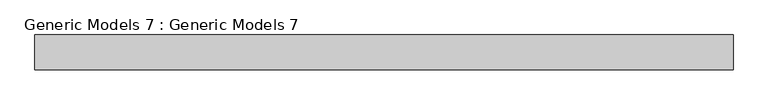
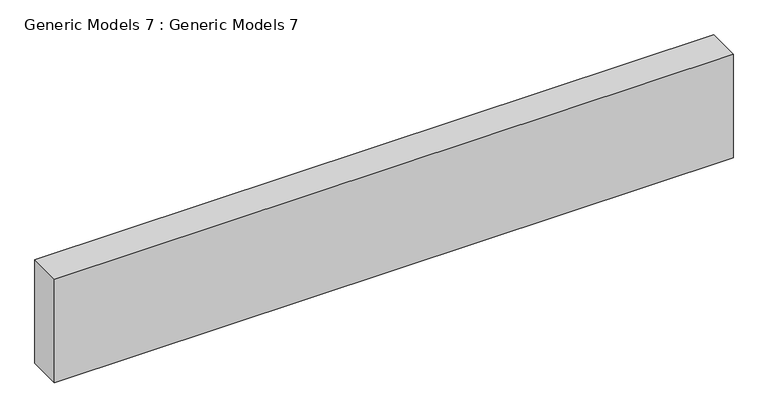
"""IFC4 building model written with IfcOpenShell, lengths in millimetres: proxy geometry, Generic Models 7 : Generic Models 7."""

from ifc_helpers import new_model, si_unit, frame, origin, place, context, project, spatial, polyline, outline, extrude, source, transform, mapped, element, save


def generic_models_7_generic_models_7_f087c847(model_context):
    return source(origin(), model_context, "Body", "SweptSolid", [
        extrude(outline(polyline([(-7615.5503587, -13873.3526331), (-12187.5503587, -13873.3526331), (-12187.5503587, -13644.7526331), (-7615.5503587, -13644.7526331), (-7615.5503587, -13873.3526331)])), frame((0.0, 0.0, 6400.8), z_axis=(0.0, 0.0, 1.0), x_axis=(1.0, 0.0, 0.0)), (0.0, 0.0, 1.0), 737.5181991),
    ])


if __name__ == "__main__":
    model = new_model("IFC4")
    model_context = context("Model", 3, world=origin())
    ifc_project = project(units=[si_unit("LENGTHUNIT", "METRE", prefix="MILLI")], contexts=[model_context])
    site = spatial("IfcSite", under=ifc_project)
    building = spatial("IfcBuilding", under=site)
    placement = place(None, origin())
    generic_models_7_generic_models_7_shape = generic_models_7_generic_models_7_f087c847(model_context)
    element("IfcBuildingElementProxy", 1, Name="Generic Models 7 : Generic Models 7", ObjectType="Generic Models 7 : Generic Models 7", at=placement, inside=building, context=model_context, shape_type="MappedRepresentation", body=[
        mapped(generic_models_7_generic_models_7_shape, transform((0.0, 0.0, 0.0), x_axis=(1.0, 0.0, 0.0), y_axis=(0.0, 1.0, 0.0), z_axis=(0.0, 0.0, 1.0))),
    ])
    save(model, "model.ifc")
